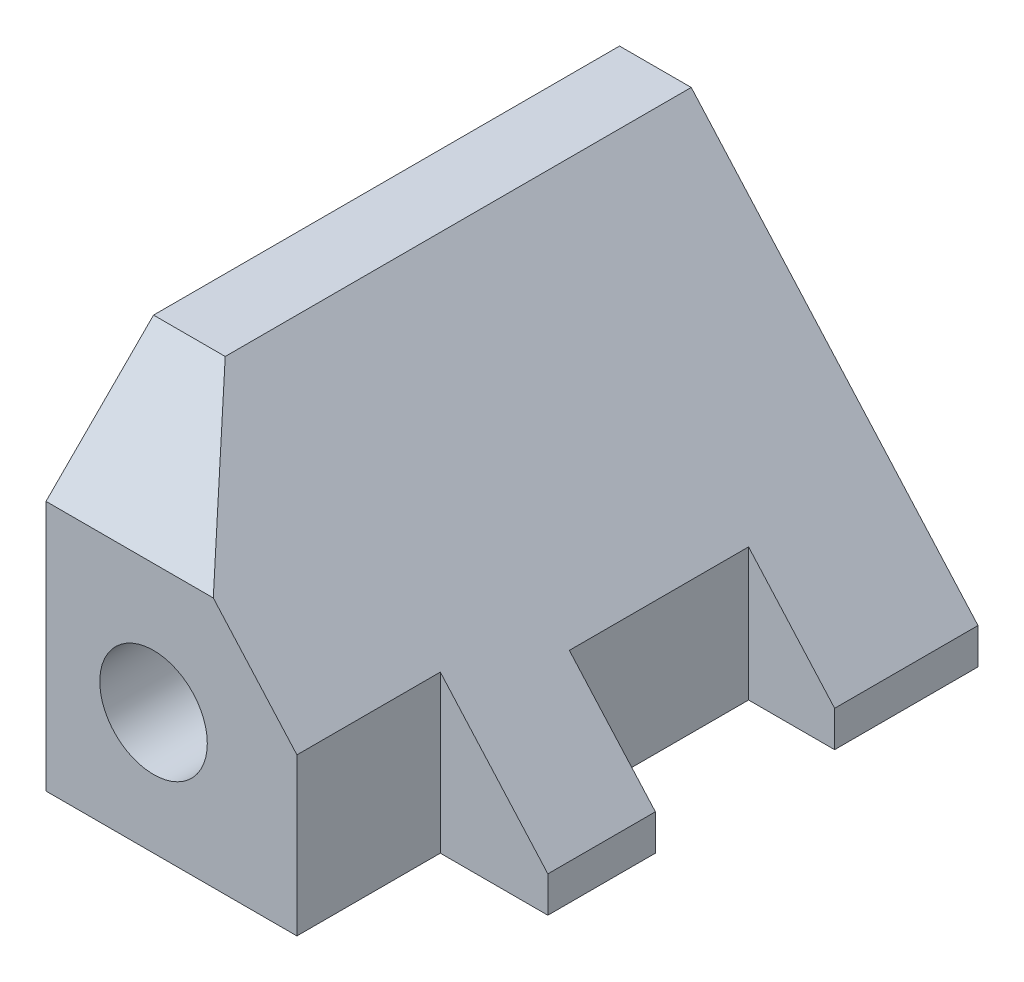
ISO-10303-21;
HEADER;
FILE_DESCRIPTION(('STEP AP214'),'2;1');
FILE_NAME('part.step','',(''),(''),'','','');
FILE_SCHEMA(('AUTOMOTIVE_DESIGN { 1 0 10303 214 1 1 1 1 }'));
ENDSEC;
DATA;
#1=APPLICATION_CONTEXT('core data for automotive mechanical design processes');
#2=APPLICATION_PROTOCOL_DEFINITION('international standard','automotive_design',2000,#1);
#3=PRODUCT_CONTEXT('',#1,'mechanical');
#4=PRODUCT('Part','Part','',(#3));
#5=PRODUCT_RELATED_PRODUCT_CATEGORY('part','',(#4));
#6=PRODUCT_DEFINITION_FORMATION('','',#4);
#7=PRODUCT_DEFINITION_CONTEXT('part definition',#1,'design');
#8=PRODUCT_DEFINITION('design','',#6,#7);
#9=PRODUCT_DEFINITION_SHAPE('','',#8);
#10=(LENGTH_UNIT() NAMED_UNIT(*) SI_UNIT(.MILLI.,.METRE.));
#11=(NAMED_UNIT(*) PLANE_ANGLE_UNIT() SI_UNIT($,.RADIAN.));
#12=(NAMED_UNIT(*) SI_UNIT($,.STERADIAN.) SOLID_ANGLE_UNIT());
#13=UNCERTAINTY_MEASURE_WITH_UNIT(LENGTH_MEASURE(1.E-05),#10,'distance_accuracy_value','');
#14=(GEOMETRIC_REPRESENTATION_CONTEXT(3) GLOBAL_UNCERTAINTY_ASSIGNED_CONTEXT((#13)) GLOBAL_UNIT_ASSIGNED_CONTEXT((#10,
#11,#12)) REPRESENTATION_CONTEXT('',''));
#15=CARTESIAN_POINT('',(0.,0.,0.));
#16=DIRECTION('',(0.,0.,1.));
#17=DIRECTION('',(1.,0.,0.));
#18=AXIS2_PLACEMENT_3D('',#15,#16,#17);
#19=CARTESIAN_POINT('',(0.,0.,80.));
#20=DIRECTION('',(0.,0.,1.));
#21=DIRECTION('',(1.,0.,0.));
#22=AXIS2_PLACEMENT_3D('',#19,#20,#21);
#23=PLANE('',#22);
#24=CARTESIAN_POINT('',(15.,17.,80.));
#25=DIRECTION('',(0.,0.,1.));
#26=DIRECTION('',(1.,0.,0.));
#27=AXIS2_PLACEMENT_3D('',#24,#25,#26);
#28=CIRCLE('',#27,7.5);
#29=CARTESIAN_POINT('',(22.5,17.,80.));
#30=VERTEX_POINT('',#29);
#31=EDGE_CURVE('E244',#30,#30,#28,.T.);
#32=ORIENTED_EDGE('',*,*,#31,.F.);
#33=EDGE_LOOP('',(#32));
#34=FACE_BOUND('',#33,.T.);
#35=DIRECTION('',(-0.66436383882992,0.74740931868366,0.));
#36=VECTOR('',#35,1.);
#37=CARTESIAN_POINT('',(50.,5.,80.));
#38=LINE('',#37,#36);
#39=CARTESIAN_POINT('',(35.,21.875,80.));
#40=VERTEX_POINT('',#39);
#41=CARTESIAN_POINT('',(23.3333333333333,35.,80.));
#42=VERTEX_POINT('',#41);
#43=EDGE_CURVE('E151',#40,#42,#38,.T.);
#44=ORIENTED_EDGE('',*,*,#43,.T.);
#45=DIRECTION('',(-1.,0.,0.));
#46=VECTOR('',#45,1.);
#47=CARTESIAN_POINT('',(0.,35.,80.));
#48=LINE('',#47,#46);
#49=CARTESIAN_POINT('',(0.,35.,80.));
#50=VERTEX_POINT('',#49);
#51=EDGE_CURVE('E11',#42,#50,#48,.T.);
#52=ORIENTED_EDGE('',*,*,#51,.T.);
#53=DIRECTION('',(0.,-1.,0.));
#54=VECTOR('',#53,1.);
#55=CARTESIAN_POINT('',(0.,50.,80.));
#56=LINE('',#55,#54);
#57=CARTESIAN_POINT('',(0.,0.,80.));
#58=VERTEX_POINT('',#57);
#59=EDGE_CURVE('E144',#50,#58,#56,.T.);
#60=ORIENTED_EDGE('',*,*,#59,.T.);
#61=DIRECTION('',(1.,0.,0.));
#62=VECTOR('',#61,1.);
#63=CARTESIAN_POINT('',(0.,0.,80.));
#64=LINE('',#63,#62);
#65=CARTESIAN_POINT('',(35.,0.,80.));
#66=VERTEX_POINT('',#65);
#67=EDGE_CURVE('E159',#58,#66,#64,.T.);
#68=ORIENTED_EDGE('',*,*,#67,.T.);
#69=DIRECTION('',(0.,-1.,0.));
#70=VECTOR('',#69,1.);
#71=CARTESIAN_POINT('',(35.,0.,80.));
#72=LINE('',#71,#70);
#73=EDGE_CURVE('E169',#40,#66,#72,.T.);
#74=ORIENTED_EDGE('',*,*,#73,.F.);
#75=EDGE_LOOP('',(#44,#52,#60,#68,#74));
#76=FACE_BOUND('',#75,.T.);
#77=ADVANCED_FACE('F43',(#34,#76),#23,.T.);
#78=CARTESIAN_POINT('',(50.,0.,80.));
#79=DIRECTION('',(-1.,0.,0.));
#80=DIRECTION('',(0.,0.,1.));
#81=AXIS2_PLACEMENT_3D('',#78,#79,#80);
#82=PLANE('',#81);
#83=DIRECTION('',(0.,0.,-1.));
#84=VECTOR('',#83,1.);
#85=CARTESIAN_POINT('',(50.,5.,80.));
#86=LINE('',#85,#84);
#87=CARTESIAN_POINT('',(50.,5.00000000000002,20.));
#88=VERTEX_POINT('',#87);
#89=CARTESIAN_POINT('',(50.,5.,0.));
#90=VERTEX_POINT('',#89);
#91=EDGE_CURVE('E152',#88,#90,#86,.T.);
#92=ORIENTED_EDGE('',*,*,#91,.F.);
#93=DIRECTION('',(0.,-1.,0.));
#94=VECTOR('',#93,1.);
#95=CARTESIAN_POINT('',(50.,80.,20.));
#96=LINE('',#95,#94);
#97=CARTESIAN_POINT('',(50.,0.,20.));
#98=VERTEX_POINT('',#97);
#99=EDGE_CURVE('E209',#88,#98,#96,.T.);
#100=ORIENTED_EDGE('',*,*,#99,.T.);
#101=DIRECTION('',(0.,0.,-1.));
#102=VECTOR('',#101,1.);
#103=CARTESIAN_POINT('',(50.,0.,80.));
#104=LINE('',#103,#102);
#105=CARTESIAN_POINT('',(50.,0.,0.));
#106=VERTEX_POINT('',#105);
#107=EDGE_CURVE('E161',#98,#106,#104,.T.);
#108=ORIENTED_EDGE('',*,*,#107,.T.);
#109=DIRECTION('',(0.,1.,0.));
#110=VECTOR('',#109,1.);
#111=CARTESIAN_POINT('',(50.,0.,0.));
#112=LINE('',#111,#110);
#113=EDGE_CURVE('E227',#106,#90,#112,.T.);
#114=ORIENTED_EDGE('',*,*,#113,.T.);
#115=EDGE_LOOP('',(#92,#100,#108,#114));
#116=FACE_BOUND('',#115,.T.);
#117=ADVANCED_FACE('F277',(#116),#82,.F.);
#118=CARTESIAN_POINT('',(0.,50.,80.));
#119=DIRECTION('',(1.,0.,0.));
#120=DIRECTION('',(0.,0.,-1.));
#121=AXIS2_PLACEMENT_3D('',#118,#119,#120);
#122=PLANE('',#121);
#123=ORIENTED_EDGE('',*,*,#59,.F.);
#124=DIRECTION('',(0.,-0.707106781186544,0.707106781186551));
#125=VECTOR('',#124,1.);
#126=CARTESIAN_POINT('',(0.,35.,80.));
#127=LINE('',#126,#125);
#128=CARTESIAN_POINT('',(0.,50.,64.9999999999998));
#129=VERTEX_POINT('',#128);
#130=EDGE_CURVE('E56',#129,#50,#127,.T.);
#131=ORIENTED_EDGE('',*,*,#130,.F.);
#132=DIRECTION('',(0.,0.,-1.));
#133=VECTOR('',#132,1.);
#134=CARTESIAN_POINT('',(0.,50.,80.));
#135=LINE('',#134,#133);
#136=CARTESIAN_POINT('',(0.,50.,0.));
#137=VERTEX_POINT('',#136);
#138=EDGE_CURVE('E142',#129,#137,#135,.T.);
#139=ORIENTED_EDGE('',*,*,#138,.T.);
#140=DIRECTION('',(0.,-1.,0.));
#141=VECTOR('',#140,1.);
#142=CARTESIAN_POINT('',(0.,50.,0.));
#143=LINE('',#142,#141);
#144=CARTESIAN_POINT('',(0.,0.,0.));
#145=VERTEX_POINT('',#144);
#146=EDGE_CURVE('E218',#137,#145,#143,.T.);
#147=ORIENTED_EDGE('',*,*,#146,.T.);
#148=DIRECTION('',(0.,0.,-1.));
#149=VECTOR('',#148,1.);
#150=CARTESIAN_POINT('',(0.,0.,80.));
#151=LINE('',#150,#149);
#152=EDGE_CURVE('E168',#58,#145,#151,.T.);
#153=ORIENTED_EDGE('',*,*,#152,.F.);
#154=EDGE_LOOP('',(#123,#131,#139,#147,#153));
#155=FACE_BOUND('',#154,.T.);
#156=ADVANCED_FACE('F44',(#155),#122,.F.);
#157=CARTESIAN_POINT('',(0.,0.,80.));
#158=DIRECTION('',(0.,1.,0.));
#159=DIRECTION('',(0.,0.,1.));
#160=AXIS2_PLACEMENT_3D('',#157,#158,#159);
#161=PLANE('',#160);
#162=CARTESIAN_POINT('',(50.,0.,60.));
#163=VERTEX_POINT('',#162);
#164=CARTESIAN_POINT('',(50.,0.,45.));
#165=VERTEX_POINT('',#164);
#166=EDGE_CURVE('E164',#163,#165,#104,.T.);
#167=ORIENTED_EDGE('',*,*,#166,.F.);
#168=DIRECTION('',(1.,0.,0.));
#169=VECTOR('',#168,1.);
#170=CARTESIAN_POINT('',(50.,0.,60.));
#171=LINE('',#170,#169);
#172=CARTESIAN_POINT('',(35.,0.,60.));
#173=VERTEX_POINT('',#172);
#174=EDGE_CURVE('E254',#173,#163,#171,.T.);
#175=ORIENTED_EDGE('',*,*,#174,.F.);
#176=DIRECTION('',(0.,0.,-1.));
#177=VECTOR('',#176,1.);
#178=CARTESIAN_POINT('',(35.,0.,80.));
#179=LINE('',#178,#177);
#180=EDGE_CURVE('E220',#66,#173,#179,.T.);
#181=ORIENTED_EDGE('',*,*,#180,.F.);
#182=ORIENTED_EDGE('',*,*,#67,.F.);
#183=ORIENTED_EDGE('',*,*,#152,.T.);
#184=DIRECTION('',(1.,0.,0.));
#185=VECTOR('',#184,1.);
#186=CARTESIAN_POINT('',(0.,0.,0.));
#187=LINE('',#186,#185);
#188=EDGE_CURVE('E223',#145,#106,#187,.T.);
#189=ORIENTED_EDGE('',*,*,#188,.T.);
#190=ORIENTED_EDGE('',*,*,#107,.F.);
#191=DIRECTION('',(1.,0.,0.));
#192=VECTOR('',#191,1.);
#193=CARTESIAN_POINT('',(50.,0.,20.));
#194=LINE('',#193,#192);
#195=CARTESIAN_POINT('',(38.,0.,20.));
#196=VERTEX_POINT('',#195);
#197=EDGE_CURVE('E197',#196,#98,#194,.T.);
#198=ORIENTED_EDGE('',*,*,#197,.F.);
#199=DIRECTION('',(0.,0.,-1.));
#200=VECTOR('',#199,1.);
#201=CARTESIAN_POINT('',(38.,0.,45.));
#202=LINE('',#201,#200);
#203=CARTESIAN_POINT('',(38.,0.,45.));
#204=VERTEX_POINT('',#203);
#205=EDGE_CURVE('E199',#204,#196,#202,.T.);
#206=ORIENTED_EDGE('',*,*,#205,.F.);
#207=DIRECTION('',(-1.,0.,0.));
#208=VECTOR('',#207,1.);
#209=CARTESIAN_POINT('',(50.,0.,45.));
#210=LINE('',#209,#208);
#211=EDGE_CURVE('E213',#165,#204,#210,.T.);
#212=ORIENTED_EDGE('',*,*,#211,.F.);
#213=EDGE_LOOP('',(#167,#175,#181,#182,#183,#189,#190,#198,#206,#212));
#214=FACE_BOUND('',#213,.T.);
#215=ADVANCED_FACE('F238',(#214),#161,.F.);
#216=CARTESIAN_POINT('',(50.,5.00000000000002,60.));
#217=VERTEX_POINT('',#216);
#218=CARTESIAN_POINT('',(50.,5.00000000000002,45.));
#219=VERTEX_POINT('',#218);
#220=EDGE_CURVE('E162',#217,#219,#86,.T.);
#221=ORIENTED_EDGE('',*,*,#220,.F.);
#222=DIRECTION('',(0.,-1.,0.));
#223=VECTOR('',#222,1.);
#224=CARTESIAN_POINT('',(50.,80.,60.));
#225=LINE('',#224,#223);
#226=EDGE_CURVE('E191',#217,#163,#225,.T.);
#227=ORIENTED_EDGE('',*,*,#226,.T.);
#228=ORIENTED_EDGE('',*,*,#166,.T.);
#229=DIRECTION('',(0.,-1.,0.));
#230=VECTOR('',#229,1.);
#231=CARTESIAN_POINT('',(50.,80.,45.));
#232=LINE('',#231,#230);
#233=EDGE_CURVE('E196',#219,#165,#232,.T.);
#234=ORIENTED_EDGE('',*,*,#233,.F.);
#235=EDGE_LOOP('',(#221,#227,#228,#234));
#236=FACE_BOUND('',#235,.T.);
#237=ADVANCED_FACE('F195',(#236),#82,.F.);
#238=CARTESIAN_POINT('',(50.,5.,80.));
#239=DIRECTION('',(-0.74740931868366,-0.66436383882992,0.));
#240=DIRECTION('',(0.66436383882992,-0.74740931868366,0.));
#241=AXIS2_PLACEMENT_3D('',#238,#239,#240);
#242=PLANE('',#241);
#243=DIRECTION('',(0.,0.,-1.));
#244=VECTOR('',#243,1.);
#245=CARTESIAN_POINT('',(10.,50.,80.));
#246=LINE('',#245,#244);
#247=CARTESIAN_POINT('',(10.,50.,64.9999999999998));
#248=VERTEX_POINT('',#247);
#249=CARTESIAN_POINT('',(10.,50.,0.));
#250=VERTEX_POINT('',#249);
#251=EDGE_CURVE('E148',#248,#250,#246,.T.);
#252=ORIENTED_EDGE('',*,*,#251,.F.);
#253=DIRECTION('',(0.53215208419019,-0.598671094713963,0.598671094713969));
#254=VECTOR('',#253,1.);
#255=CARTESIAN_POINT('',(40.4424778761061,15.7522123893807,99.2477876106195));
#256=LINE('',#255,#254);
#257=EDGE_CURVE('E132',#248,#42,#256,.T.);
#258=ORIENTED_EDGE('',*,*,#257,.T.);
#259=ORIENTED_EDGE('',*,*,#43,.F.);
#260=DIRECTION('',(0.,0.,-1.));
#261=VECTOR('',#260,1.);
#262=CARTESIAN_POINT('',(35.,21.875,80.));
#263=LINE('',#262,#261);
#264=CARTESIAN_POINT('',(35.,21.875,60.));
#265=VERTEX_POINT('',#264);
#266=EDGE_CURVE('E187',#40,#265,#263,.T.);
#267=ORIENTED_EDGE('',*,*,#266,.T.);
#268=DIRECTION('',(0.66436383882992,-0.74740931868366,0.));
#269=VECTOR('',#268,1.);
#270=CARTESIAN_POINT('',(50.,5.,60.));
#271=LINE('',#270,#269);
#272=EDGE_CURVE('E55',#265,#217,#271,.T.);
#273=ORIENTED_EDGE('',*,*,#272,.T.);
#274=ORIENTED_EDGE('',*,*,#220,.T.);
#275=DIRECTION('',(-0.66436383882992,0.74740931868366,0.));
#276=VECTOR('',#275,1.);
#277=CARTESIAN_POINT('',(50.,5.,45.));
#278=LINE('',#277,#276);
#279=CARTESIAN_POINT('',(38.,18.5,45.));
#280=VERTEX_POINT('',#279);
#281=EDGE_CURVE('E171',#219,#280,#278,.T.);
#282=ORIENTED_EDGE('',*,*,#281,.T.);
#283=DIRECTION('',(0.,0.,-1.));
#284=VECTOR('',#283,1.);
#285=CARTESIAN_POINT('',(38.,18.5,80.));
#286=LINE('',#285,#284);
#287=CARTESIAN_POINT('',(38.,18.5,20.));
#288=VERTEX_POINT('',#287);
#289=EDGE_CURVE('E172',#280,#288,#286,.T.);
#290=ORIENTED_EDGE('',*,*,#289,.T.);
#291=DIRECTION('',(0.66436383882992,-0.74740931868366,0.));
#292=VECTOR('',#291,1.);
#293=CARTESIAN_POINT('',(50.,5.,20.));
#294=LINE('',#293,#292);
#295=EDGE_CURVE('E180',#288,#88,#294,.T.);
#296=ORIENTED_EDGE('',*,*,#295,.T.);
#297=ORIENTED_EDGE('',*,*,#91,.T.);
#298=DIRECTION('',(-0.66436383882992,0.74740931868366,0.));
#299=VECTOR('',#298,1.);
#300=CARTESIAN_POINT('',(50.,5.,0.));
#301=LINE('',#300,#299);
#302=EDGE_CURVE('E230',#90,#250,#301,.T.);
#303=ORIENTED_EDGE('',*,*,#302,.T.);
#304=EDGE_LOOP('',(#252,#258,#259,#267,#273,#274,#282,#290,#296,#297,#303));
#305=FACE_BOUND('',#304,.T.);
#306=ADVANCED_FACE('F183',(#305),#242,.F.);
#307=CARTESIAN_POINT('',(10.,50.,80.));
#308=DIRECTION('',(0.,-1.,0.));
#309=DIRECTION('',(0.,0.,-1.));
#310=AXIS2_PLACEMENT_3D('',#307,#308,#309);
#311=PLANE('',#310);
#312=ORIENTED_EDGE('',*,*,#138,.F.);
#313=DIRECTION('',(-1.,0.,0.));
#314=VECTOR('',#313,1.);
#315=CARTESIAN_POINT('',(40.,50.,64.9999999999998));
#316=LINE('',#315,#314);
#317=EDGE_CURVE('E128',#248,#129,#316,.T.);
#318=ORIENTED_EDGE('',*,*,#317,.F.);
#319=ORIENTED_EDGE('',*,*,#251,.T.);
#320=DIRECTION('',(-1.,0.,0.));
#321=VECTOR('',#320,1.);
#322=CARTESIAN_POINT('',(10.,50.,0.));
#323=LINE('',#322,#321);
#324=EDGE_CURVE('E149',#250,#137,#323,.T.);
#325=ORIENTED_EDGE('',*,*,#324,.T.);
#326=EDGE_LOOP('',(#312,#318,#319,#325));
#327=FACE_BOUND('',#326,.T.);
#328=ADVANCED_FACE('F147',(#327),#311,.F.);
#329=CARTESIAN_POINT('',(0.,0.,0.));
#330=DIRECTION('',(0.,0.,1.));
#331=DIRECTION('',(1.,0.,0.));
#332=AXIS2_PLACEMENT_3D('',#329,#330,#331);
#333=PLANE('',#332);
#334=ORIENTED_EDGE('',*,*,#146,.F.);
#335=ORIENTED_EDGE('',*,*,#324,.F.);
#336=ORIENTED_EDGE('',*,*,#302,.F.);
#337=ORIENTED_EDGE('',*,*,#113,.F.);
#338=ORIENTED_EDGE('',*,*,#188,.F.);
#339=EDGE_LOOP('',(#334,#335,#336,#337,#338));
#340=FACE_BOUND('',#339,.T.);
#341=ADVANCED_FACE('F232',(#340),#333,.F.);
#342=CARTESIAN_POINT('',(50.,80.,60.));
#343=DIRECTION('',(0.,0.,-1.));
#344=DIRECTION('',(-1.,0.,0.));
#345=AXIS2_PLACEMENT_3D('',#342,#343,#344);
#346=PLANE('',#345);
#347=DIRECTION('',(0.,-1.,0.));
#348=VECTOR('',#347,1.);
#349=CARTESIAN_POINT('',(35.,80.,60.));
#350=LINE('',#349,#348);
#351=EDGE_CURVE('E202',#265,#173,#350,.T.);
#352=ORIENTED_EDGE('',*,*,#351,.T.);
#353=ORIENTED_EDGE('',*,*,#174,.T.);
#354=ORIENTED_EDGE('',*,*,#226,.F.);
#355=ORIENTED_EDGE('',*,*,#272,.F.);
#356=EDGE_LOOP('',(#352,#353,#354,#355));
#357=FACE_BOUND('',#356,.T.);
#358=ADVANCED_FACE('F251',(#357),#346,.F.);
#359=CARTESIAN_POINT('',(35.,80.,80.));
#360=DIRECTION('',(-1.,0.,0.));
#361=DIRECTION('',(0.,0.,1.));
#362=AXIS2_PLACEMENT_3D('',#359,#360,#361);
#363=PLANE('',#362);
#364=ORIENTED_EDGE('',*,*,#73,.T.);
#365=ORIENTED_EDGE('',*,*,#180,.T.);
#366=ORIENTED_EDGE('',*,*,#351,.F.);
#367=ORIENTED_EDGE('',*,*,#266,.F.);
#368=EDGE_LOOP('',(#364,#365,#366,#367));
#369=FACE_BOUND('',#368,.T.);
#370=ADVANCED_FACE('F257',(#369),#363,.F.);
#371=CARTESIAN_POINT('',(50.,80.,20.));
#372=DIRECTION('',(0.,0.,-1.));
#373=DIRECTION('',(-1.,0.,0.));
#374=AXIS2_PLACEMENT_3D('',#371,#372,#373);
#375=PLANE('',#374);
#376=DIRECTION('',(0.,-1.,0.));
#377=VECTOR('',#376,1.);
#378=CARTESIAN_POINT('',(38.,80.,20.));
#379=LINE('',#378,#377);
#380=EDGE_CURVE('E201',#288,#196,#379,.T.);
#381=ORIENTED_EDGE('',*,*,#380,.T.);
#382=ORIENTED_EDGE('',*,*,#197,.T.);
#383=ORIENTED_EDGE('',*,*,#99,.F.);
#384=ORIENTED_EDGE('',*,*,#295,.F.);
#385=EDGE_LOOP('',(#381,#382,#383,#384));
#386=FACE_BOUND('',#385,.T.);
#387=ADVANCED_FACE('F272',(#386),#375,.F.);
#388=CARTESIAN_POINT('',(38.,80.,45.));
#389=DIRECTION('',(-1.,0.,0.));
#390=DIRECTION('',(0.,0.,1.));
#391=AXIS2_PLACEMENT_3D('',#388,#389,#390);
#392=PLANE('',#391);
#393=DIRECTION('',(0.,-1.,0.));
#394=VECTOR('',#393,1.);
#395=CARTESIAN_POINT('',(38.,80.,45.));
#396=LINE('',#395,#394);
#397=EDGE_CURVE('E66',#280,#204,#396,.T.);
#398=ORIENTED_EDGE('',*,*,#397,.T.);
#399=ORIENTED_EDGE('',*,*,#205,.T.);
#400=ORIENTED_EDGE('',*,*,#380,.F.);
#401=ORIENTED_EDGE('',*,*,#289,.F.);
#402=EDGE_LOOP('',(#398,#399,#400,#401));
#403=FACE_BOUND('',#402,.T.);
#404=ADVANCED_FACE('F265',(#403),#392,.F.);
#405=CARTESIAN_POINT('',(50.,80.,45.));
#406=DIRECTION('',(0.,0.,1.));
#407=DIRECTION('',(1.,0.,0.));
#408=AXIS2_PLACEMENT_3D('',#405,#406,#407);
#409=PLANE('',#408);
#410=ORIENTED_EDGE('',*,*,#233,.T.);
#411=ORIENTED_EDGE('',*,*,#211,.T.);
#412=ORIENTED_EDGE('',*,*,#397,.F.);
#413=ORIENTED_EDGE('',*,*,#281,.F.);
#414=EDGE_LOOP('',(#410,#411,#412,#413));
#415=FACE_BOUND('',#414,.T.);
#416=ADVANCED_FACE('F256',(#415),#409,.F.);
#417=CARTESIAN_POINT('',(15.,17.,40.));
#418=DIRECTION('',(0.,0.,1.));
#419=DIRECTION('',(1.,0.,0.));
#420=AXIS2_PLACEMENT_3D('',#417,#418,#419);
#421=CYLINDRICAL_SURFACE('',#420,7.5);
#422=CARTESIAN_POINT('',(15.,17.,40.));
#423=DIRECTION('',(0.,0.,1.));
#424=DIRECTION('',(1.,0.,0.));
#425=AXIS2_PLACEMENT_3D('',#422,#423,#424);
#426=CIRCLE('',#425,7.5);
#427=CARTESIAN_POINT('',(22.5,17.,40.));
#428=VERTEX_POINT('',#427);
#429=EDGE_CURVE('E212',#428,#428,#426,.T.);
#430=ORIENTED_EDGE('',*,*,#429,.F.);
#431=EDGE_LOOP('',(#430));
#432=FACE_BOUND('',#431,.T.);
#433=ORIENTED_EDGE('',*,*,#31,.T.);
#434=EDGE_LOOP('',(#433));
#435=FACE_BOUND('',#434,.T.);
#436=ADVANCED_FACE('F261',(#432,#435),#421,.F.);
#437=CARTESIAN_POINT('',(15.,17.,40.));
#438=DIRECTION('',(0.,0.,1.));
#439=DIRECTION('',(1.,0.,0.));
#440=AXIS2_PLACEMENT_3D('',#437,#438,#439);
#441=PLANE('',#440);
#442=ORIENTED_EDGE('',*,*,#429,.T.);
#443=EDGE_LOOP('',(#442));
#444=FACE_BOUND('',#443,.T.);
#445=ADVANCED_FACE('F270',(#444),#441,.T.);
#446=CARTESIAN_POINT('',(40.,35.,80.));
#447=DIRECTION('',(0.,-0.707106781186551,-0.707106781186544));
#448=DIRECTION('',(0.,0.707106781186544,-0.707106781186551));
#449=AXIS2_PLACEMENT_3D('',#446,#447,#448);
#450=PLANE('',#449);
#451=ORIENTED_EDGE('',*,*,#317,.T.);
#452=ORIENTED_EDGE('',*,*,#130,.T.);
#453=ORIENTED_EDGE('',*,*,#51,.F.);
#454=ORIENTED_EDGE('',*,*,#257,.F.);
#455=EDGE_LOOP('',(#451,#452,#453,#454));
#456=FACE_BOUND('',#455,.T.);
#457=ADVANCED_FACE('F131',(#456),#450,.F.);
#458=CLOSED_SHELL('',(#77,#117,#156,#215,#237,#306,#328,#341,#358,#370,#387,#404,#416,#436,#445,#457));
#459=MANIFOLD_SOLID_BREP('B2',#458);
#460=ADVANCED_BREP_SHAPE_REPRESENTATION('',(#18,#459),#14);
#461=SHAPE_DEFINITION_REPRESENTATION(#9,#460);
ENDSEC;
END-ISO-10303-21;
